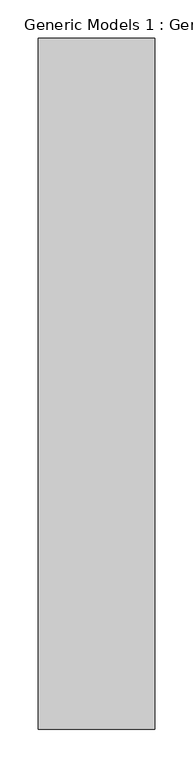
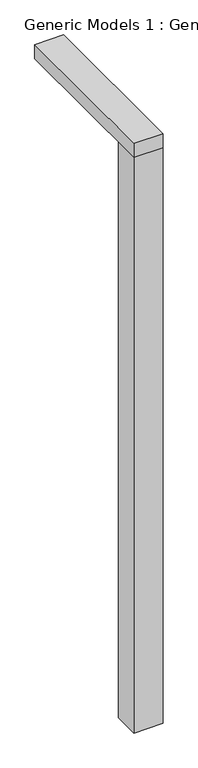
"""IFC4 building model written with IfcOpenShell, lengths in millimetres: proxy geometry, Generic Models 1 : Generic Models 1."""

from ifc_helpers import new_model, si_unit, frame, origin, origin_with_axes, place, context, project, spatial, polyline, outline, extrude, source, transform, mapped, element, save


def generic_models_1_generic_models_1_a0d4ce11(model_context):
    return source(origin(), model_context, "Body", "SweptSolid", [
        extrude(outline(polyline([(-9698.5642415, -4709.7273102), (-9546.1642415, -4709.7273102), (-9546.1642415, -5613.7098142), (-9698.5642415, -5613.7098142), (-9698.5642415, -4709.7273102)])), frame((0.0, 0.0, 3200.4), z_axis=(0.0, 0.0, 1.0), x_axis=(1.0, 0.0, 0.0)), (0.0, 0.0, 1.0), 79.9931522),
        extrude(outline(polyline([(-9698.5642415, -5471.7273102), (-9546.1642415, -5471.7273102), (-9546.1642415, -5613.7098142), (-9698.5642415, -5613.7098142), (-9698.5642415, -5471.7273102)])), origin_with_axes(), (0.0, 0.0, 1.0), 3200.4),
    ])


if __name__ == "__main__":
    model = new_model("IFC4")
    model_context = context("Model", 3, world=origin())
    ifc_project = project(units=[si_unit("LENGTHUNIT", "METRE", prefix="MILLI")], contexts=[model_context])
    site = spatial("IfcSite", under=ifc_project)
    building = spatial("IfcBuilding", under=site)
    placement = place(None, origin())
    generic_models_1_generic_models_1_shape = generic_models_1_generic_models_1_a0d4ce11(model_context)
    element("IfcBuildingElementProxy", 1, Name="Generic Models 1 : Generic Models 1", ObjectType="Generic Models 1 : Generic Models 1", at=placement, inside=building, context=model_context, shape_type="MappedRepresentation", body=[
        mapped(generic_models_1_generic_models_1_shape, transform((0.0, 0.0, 0.0), x_axis=(1.0, 0.0, 0.0), y_axis=(0.0, 1.0, 0.0), z_axis=(0.0, 0.0, 1.0))),
    ])
    save(model, "model.ifc")

# Revit data of these elements
# Element 1 (IfcBuildingElementProxy, "Generic Models 1 : Generic Models 1")
#   Materials on its faces: "exterior wall"
# Materials
#   "exterior wall": class "Generic", colour RGB 215 217 121, transparency 0, Cost = 0
